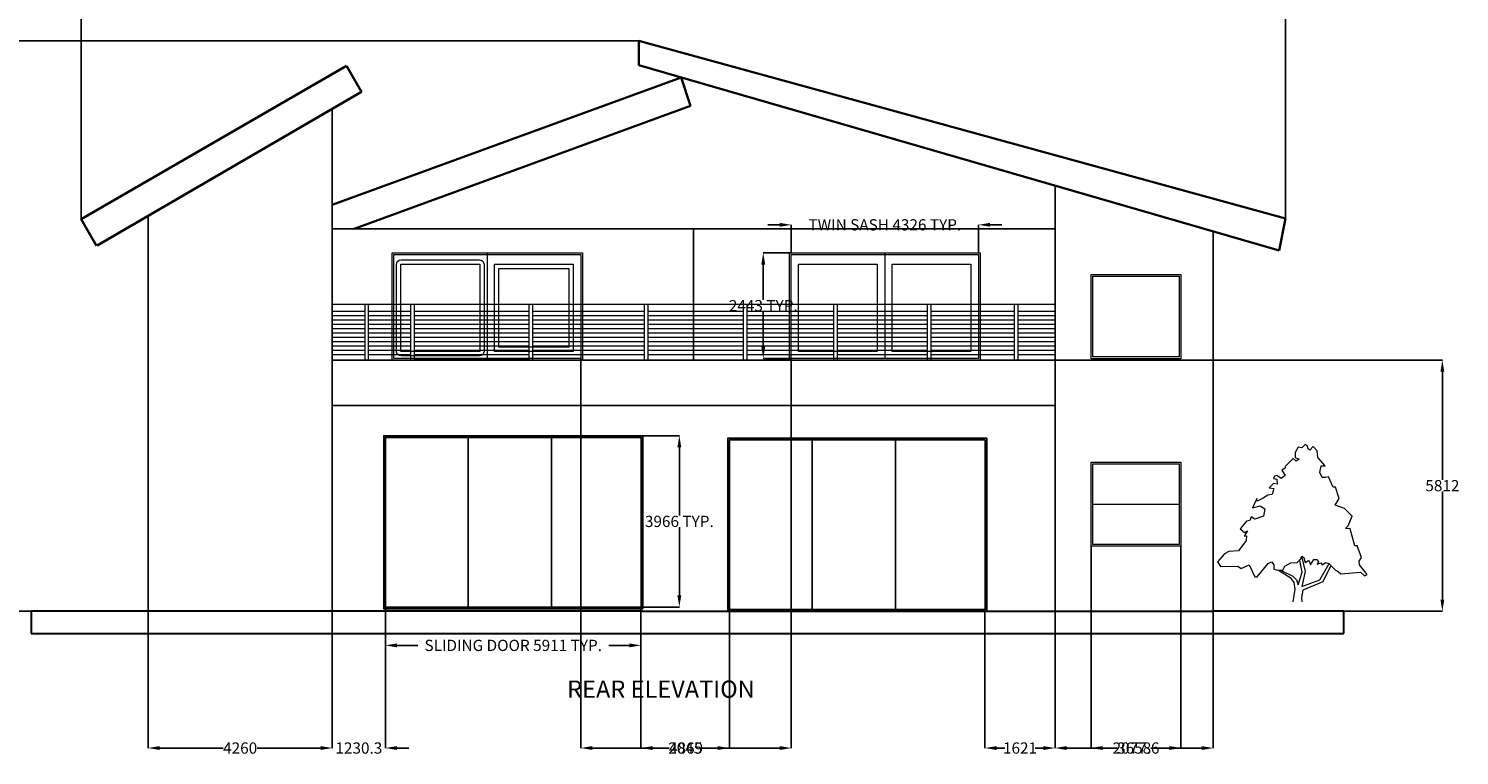
# Model space of a CAD drawing. Units: millimetres. Extents: x 23 to 3809233, y 4 to 290343.
# Tile 5 of 8: x 1915648 to 1948739, y 132658 to 149481. Entities that reach past the tile are written whole.
import ezdxf

# ---------------------------------------------------------------- set-up
doc = ezdxf.new("R2010")
doc.units = ezdxf.units.MM
doc.header["$MEASUREMENT"] = 0
for name, color, linetype, lineweight in [('A-ANNO-DIMS', 2, 'Continuous', 18), ('A-ANNO-TEXT', 7, 'Continuous', 25), ('A-DOOR', 3, 'Continuous', 25), ('A-ELEV', 7, 'Continuous', 25), ('A-ELEV-GRND', 7, 'Continuous', 30), ('A-FLOR-RAIL', 8, 'Continuous', 18), ('A-GLAZ', 4, 'Continuous', 18), ('A-ROOF', 7, 'Continuous', 35), ('L-PLNT', 94, 'Continuous', 13)]:
    doc.layers.add(name, color=color, linetype=linetype, lineweight=lineweight)
doc.styles.get("Standard").update_dxf_attribs({"font": 'arial.ttf'})
doc.dimstyles.get("Standard").update_dxf_attribs({"dimtxt": 260.18, "dimasz": 270.18, "dimexe": 0.18, "dimexo": 0.0625, "dimgap": 0.09, "dimtad": 0, "dimtih": 1, "dimtoh": 1, "dimdec": 0, "dimzin": 0, "dimdsep": 46, "dimtxsty": 'Standard', "dimcen": 0.09, "dimadec": 0, "dimazin": 0, "dimtfac": 1, "dimtdec": 0, "dimtofl": 0, "dimtmove": 0, "dimatfit": 3, "dimfxl": 1, "dimtolj": 1, "dimtzin": 0, "dimarcsym": 0})

# ---------------------------------------------------------------- blocks, each defined once
blk = doc.blocks.new('*U4')
for points in [[(22.0124, 137.721), (18.5475, 141.5624), (15.5282, 138.2446), (13.8028, 139.3505), (13.3714, 142.1153), (11.2148, 143.2214), (8.1954, 140.4564), (4.7447, 141.0094), (2.1567, 136.0326), (2.1567, 131.6088), (5.6074, 129.9499), (3.0193, 128.2909), (0.4313, 130.5029), (-6.9015, 123.3141), (-6.9015, 121.6552), (-9.9208, 119.9963), (-9.0581, 118.3373), (-6.9015, 115.0195), (-10.7835, 112.2546), (-14.6656, 115.0195), (-16.8222, 114.4665), (-17.6849, 112.2546), (-14.6656, 111.7016), (-14.2342, 107.2778), (-17.6065, 107.8307), (-21.5669, 103.9599), (-17.2536, 103.4069), (-18.9789, 97.8771), (-22.8609, 97.3241), (-27.1743, 94.5593), (-32.3504, 91.7944), (-32.7817, 94.0063), (-36.6638, 85.7116), (-29.7624, 87.3705), (-25.449, 84.6056), (-26.743, 77.9699), (-34.507, 75.205), (-37.9578, 77.4169), (-39.2518, 74.099), (-42.2711, 73.5461), (-44.8592, 70.2282), (-47.8786, 66.3574), (-43.9965, 63.0395), (-41.4085, 64.6985), (-44.3346, 59.8898), (-42.2089, 60.1377), (-42.5159, 55.7849), (-49.6039, 46.4502), (-58.2307, 45.8972), (-62.1127, 43.6853), (-68.5828, 36.4966), (-65.9947, 32.0727), (-50.0352, 32.6257), (-47.0159, 30.4138), (-39.6831, 33.7317), (-34.507, 22.6721), (-32.3504, 22.6721), (-22.4296, 34.8376), (-19.4102, 36.4966), (-17.2536, 33.7317), (-17.2536, 29.8608), (-13.8028, 28.7549), (-9.0581, 28.7549), (-7.3328, 32.6257), (-1.7254, 35.3906), (3.8821, 35.9436), (6.4701, 38.1555), (6.9014, 38.7085), (8.1954, 41.4734), (9.9208, 40.3674), (11.2148, 35.9436), (14.2341, 37.6025), (15.0968, 36.4966), (15.9595, 33.7317), (18.9789, 38.7085), (21.9982, 38.7085), (23.2922, 36.4966), (21.9982, 34.2847), (25.4489, 35.3906), (26.743, 33.7317), (29.7623, 35.9436), (32.7817, 34.8376), (38.8204, 28.7549), (41.4084, 27.6489), (43.5651, 25.437), (61.6813, 27.0959), (65.132, 23.7781), (67.7201, 24.884), (60.8186, 33.7317), (60.3873, 37.0495), (62.544, 40.3674), (58.662, 50.874), (56.5053, 50.874), (52.1919, 66.3574), (47.8785, 66.9103), (50.4665, 69.1222), (53.9172, 77.9699), (47.0158, 85.1586), (38.3891, 87.9235), (42.2711, 94.0063)], [(42.2711, 94.0063), (38.8204, 104.5129), (36.6637, 104.5129), (32.3503, 113.9135), (29.7623, 113.3605), (26.743, 113.3605), (24.5862, 117.7844), (25.8802, 123.8671), (29.331, 123.8671), (22.8609, 131.6088), (21.9982, 137.6916)], [(8.1954, 40.3674), (11.2148, 27.6489), (8.1954, 13.8245), (24.5862, 19.9072), (32.7817, 34.2847)], [(-12.9401, 28.7549), (-2.588, 22.1191), (0.8626, 17.6953), (1.7253, 11.6125), (0, 0)], [(-9.9208, 28.2019), (0, 23.2251), (3.4507, 19.9072), (4.7447, 15.4834), (8.6267, 27.0959), (6.4701, 37.6025)], [(34.5071, 33.1787), (27.1743, 18.2483), (9.0581, 10.5066), (7.7641, 3.8708), (8.1954, 0)]]:
    blk.add_lwpolyline(points)
blk = doc.blocks.new('WINDOW-TWIN-SASH-ELEV')
blk.add_line((2163, 2443), (2163, 0))
blk.add_lwpolyline([(0, 2403), (4326, 2403), (4326, 0), (0, 0)], close=True)
for points in [[(165, 2176, -0.414214), (168, 2179), (1985, 2179, -0.414214), (1988, 2176), (1988, 160, -0.414214), (1985, 157), (168, 157, -0.414214), (165, 160)], [(2329, 2176, -0.414214), (2332, 2179), (4148, 2179, -0.414214), (4151, 2176), (4151, 160, -0.414214), (4148, 157), (2332, 157, -0.414214), (2329, 160)]]:
    blk.add_lwpolyline(points, format="xyb", close=True)
blk = doc.blocks.new('SLIDER-THREE-PANEL-ELEV')
for p, q in [((1912, 3966), (1912, 0)), ((3839, 3926), (3839, 0))]:
    blk.add_line(p, q)
blk.add_lwpolyline([(5911, 0), (0, 0), (0, 3926), (5911, 3926)], close=True)
blk = doc.blocks.new('*D44')
at = {"layer": 'A-ANNO-DIMS', "color": 0, "lineweight": -2, "transparency": 16777216}
for p, q in [((1933018, 144939), (1932747, 144939)), ((1933288, 144290), (1933288, 144939)), ((1937614, 144290), (1937614, 144939)), ((1937884, 144939), (1938154, 144939))]:
    blk.add_line(p, q, dxfattribs=at)
at = {"layer": 'A-ANNO-DIMS', "color": 0, "transparency": 16777216}
for points in [[(1933018, 144984), (1933018, 144894), (1933288, 144939)], [(1937884, 144984), (1937884, 144894), (1937614, 144939)]]:
    blk.add_solid(points, dxfattribs=at)
at = {"layer": 'Defpoints', "color": 0, "transparency": 16777216}
for p in [(1937614, 144939), (1933288, 144290), (1937614, 144290)]:
    blk.add_point(p, dxfattribs=at)
at = {"layer": 'A-ANNO-DIMS', "color": 0, "transparency": 16777216, "insert": (1935451, 144939), "char_height": 260.18, "attachment_point": 5}
blk.add_mtext('\\A1;TWIN SASH 4326 TYP.', dxfattribs=at)
blk = doc.blocks.new('*D45')
at = {"layer": 'A-ANNO-DIMS', "color": 0, "lineweight": -2, "transparency": 16777216}
for p, q in [((1933288, 144290), (1932639, 144290)), ((1932639, 144020), (1932639, 143202)), ((1932639, 142117), (1932639, 142935)), ((1933288, 141847), (1932639, 141847))]:
    blk.add_line(p, q, dxfattribs=at)
at = {"layer": 'A-ANNO-DIMS', "color": 0, "transparency": 16777216}
for points in [[(1932594, 144020), (1932684, 144020), (1932639, 144290)], [(1932594, 142117), (1932684, 142117), (1932639, 141847)]]:
    blk.add_solid(points, dxfattribs=at)
at = {"layer": 'Defpoints', "color": 0, "transparency": 16777216}
for p in [(1932639, 144290), (1933288, 144290), (1933288, 141847)]:
    blk.add_point(p, dxfattribs=at)
at = {"layer": 'A-ANNO-DIMS', "color": 0, "transparency": 16777216, "insert": (1932639, 143068), "char_height": 260.18, "attachment_point": 5}
blk.add_mtext('\\A1;2443 TYP.', dxfattribs=at)
blk = doc.blocks.new('*D46')
at = {"layer": 'A-ANNO-DIMS', "color": 0, "lineweight": -2, "transparency": 16777216}
for p, q in [((1923901, 136091), (1923901, 135204)), ((1929811, 136091), (1929811, 135204)), ((1924171, 135204), (1924648, 135204)), ((1929541, 135204), (1929064, 135204))]:
    blk.add_line(p, q, dxfattribs=at)
at = {"layer": 'A-ANNO-DIMS', "color": 0, "transparency": 16777216}
for points in [[(1924171, 135249), (1924171, 135159), (1923901, 135204)], [(1929541, 135249), (1929541, 135159), (1929811, 135204)]]:
    blk.add_solid(points, dxfattribs=at)
at = {"layer": 'Defpoints', "color": 0, "transparency": 16777216}
for p in [(1923901, 136091), (1929811, 136091), (1929811, 135204)]:
    blk.add_point(p, dxfattribs=at)
at = {"layer": 'A-ANNO-DIMS', "color": 0, "transparency": 16777216, "insert": (1926856, 135204), "char_height": 260.18, "attachment_point": 5}
blk.add_mtext('\\A1;SLIDING DOOR 5911 TYP.', dxfattribs=at)
blk = doc.blocks.new('*D47')
at = {"layer": 'A-ANNO-DIMS', "color": 0, "lineweight": -2, "transparency": 16777216}
for p, q in [((1929812, 140056), (1930698, 140056)), ((1930698, 139786), (1930698, 138207)), ((1930698, 136361), (1930698, 137941)), ((1929812, 136091), (1930698, 136091))]:
    blk.add_line(p, q, dxfattribs=at)
at = {"layer": 'A-ANNO-DIMS', "color": 0, "transparency": 16777216}
for points in [[(1930653, 139786), (1930743, 139786), (1930698, 140056)], [(1930653, 136361), (1930743, 136361), (1930698, 136091)]]:
    blk.add_solid(points, dxfattribs=at)
at = {"layer": 'Defpoints', "color": 0, "transparency": 16777216}
for p in [(1929811, 140056), (1930698, 140056), (1929811, 136091)]:
    blk.add_point(p, dxfattribs=at)
at = {"layer": 'A-ANNO-DIMS', "color": 0, "transparency": 16777216, "insert": (1930698, 138074), "char_height": 260.18, "attachment_point": 5}
blk.add_mtext('\\A1;3966 TYP.', dxfattribs=at)
blk = doc.blocks.new('*D116')
at = {"layer": 'A-ANNO-DIMS', "color": 0, "lineweight": -2, "transparency": 16777216}
for p, q in [((1916860, 145073), (1916860, 150759)), ((1917130, 150759), (1930297, 150759)), ((1944447, 150759), (1931281, 150759)), ((1944717, 145084), (1944717, 150759))]:
    blk.add_line(p, q, dxfattribs=at)
at = {"layer": 'A-ANNO-DIMS', "color": 0, "transparency": 16777216}
for points in [[(1917130, 150804), (1917130, 150714), (1916860, 150759)], [(1944447, 150804), (1944447, 150714), (1944717, 150759)]]:
    blk.add_solid(points, dxfattribs=at)
at = {"layer": 'Defpoints', "color": 0, "transparency": 16777216}
for p in [(1944717, 150759), (1916860, 145073), (1944717, 145084)]:
    blk.add_point(p, dxfattribs=at)
at = {"layer": 'A-ANNO-DIMS', "color": 0, "transparency": 16777216, "insert": (1930789, 150759), "char_height": 260.2, "attachment_point": 5}
blk.add_mtext('\\A1;27857', dxfattribs=at)
blk = doc.blocks.new('*D117')
at = {"layer": 'A-ANNO-DIMS', "color": 0, "lineweight": -2, "transparency": 16777216}
for p, q in [((1929762, 149200), (1914150, 149200)), ((1914150, 148930), (1914150, 142731)), ((1914150, 136265), (1914150, 142465)), ((1918411, 135995), (1914150, 135995))]:
    blk.add_line(p, q, dxfattribs=at)
at = {"layer": 'A-ANNO-DIMS', "color": 0, "transparency": 16777216}
for points in [[(1914105, 148930), (1914195, 148930), (1914150, 149200)], [(1914105, 136265), (1914195, 136265), (1914150, 135995)]]:
    blk.add_solid(points, dxfattribs=at)
at = {"layer": 'Defpoints', "color": 0, "transparency": 16777216}
for p in [(1914150, 149200), (1929762, 149200), (1918411, 135995)]:
    blk.add_point(p, dxfattribs=at)
at = {"layer": 'A-ANNO-DIMS', "color": 0, "transparency": 16777216, "insert": (1914150, 142598), "char_height": 260.2, "attachment_point": 5}
blk.add_mtext('\\A1;13205', dxfattribs=at)
blk = doc.blocks.new('*D118')
at = {"layer": 'A-ANNO-DIMS', "color": 0, "lineweight": -2, "transparency": 16777216}
for p, q in [((1918411, 135995), (1918411, 132828)), ((1922671, 135995), (1922671, 132828)), ((1918681, 132828), (1920147, 132828)), ((1922400, 132828), (1920934, 132828))]:
    blk.add_line(p, q, dxfattribs=at)
at = {"layer": 'A-ANNO-DIMS', "color": 0, "transparency": 16777216}
for points in [[(1918681, 132873), (1918681, 132783), (1918411, 132828)], [(1922400, 132873), (1922400, 132783), (1922671, 132828)]]:
    blk.add_solid(points, dxfattribs=at)
at = {"layer": 'Defpoints', "color": 0, "transparency": 16777216}
for p in [(1918411, 135995), (1922671, 135995), (1922671, 132828)]:
    blk.add_point(p, dxfattribs=at)
at = {"layer": 'A-ANNO-DIMS', "color": 0, "transparency": 16777216, "insert": (1920541, 132828), "char_height": 260.2, "attachment_point": 5}
blk.add_mtext('\\A1;4260', dxfattribs=at)
blk = doc.blocks.new('*D119')
at = {"layer": 'A-ANNO-DIMS', "color": 0, "lineweight": -2, "transparency": 16777216}
for p, q in [((1923901, 136091), (1923901, 132828)), ((1922671, 135995), (1922671, 132828)), ((1922400, 132828), (1922130, 132828)), ((1924171, 132828), (1924441, 132828))]:
    blk.add_line(p, q, dxfattribs=at)
at = {"layer": 'A-ANNO-DIMS', "color": 0, "transparency": 16777216}
for points in [[(1922400, 132873), (1922400, 132783), (1922671, 132828)], [(1924171, 132873), (1924171, 132783), (1923901, 132828)]]:
    blk.add_solid(points, dxfattribs=at)
at = {"layer": 'Defpoints', "color": 0, "transparency": 16777216}
for p in [(1923901, 136091), (1922671, 135995), (1923901, 132828)]:
    blk.add_point(p, dxfattribs=at)
at = {"layer": 'A-ANNO-DIMS', "color": 0, "transparency": 16777216, "insert": (1923286, 132828), "char_height": 260.2, "attachment_point": 5}
blk.add_mtext('\\A1;1230.3', dxfattribs=at)
blk = doc.blocks.new('*D120')
at = {"layer": 'A-ANNO-DIMS', "color": 0, "lineweight": -2, "transparency": 16777216}
for p, q in [((1929811, 136091), (1929811, 132828)), ((1931856, 136035), (1931856, 132828)), ((1930082, 132828), (1930442, 132828)), ((1931586, 132828), (1931226, 132828))]:
    blk.add_line(p, q, dxfattribs=at)
at = {"layer": 'A-ANNO-DIMS', "color": 0, "transparency": 16777216}
for points in [[(1930082, 132873), (1930082, 132783), (1929811, 132828)], [(1931586, 132873), (1931586, 132783), (1931856, 132828)]]:
    blk.add_solid(points, dxfattribs=at)
at = {"layer": 'Defpoints', "color": 0, "transparency": 16777216}
for p in [(1929811, 136091), (1931856, 136035), (1931856, 132828)]:
    blk.add_point(p, dxfattribs=at)
at = {"layer": 'A-ANNO-DIMS', "color": 0, "transparency": 16777216, "insert": (1930834, 132828), "char_height": 260.2, "attachment_point": 5}
blk.add_mtext('\\A1;2045', dxfattribs=at)
blk = doc.blocks.new('*D121')
at = {"layer": 'A-ANNO-DIMS', "color": 0, "lineweight": -2, "transparency": 16777216}
for p, q in [((1937767, 136035), (1937767, 132828)), ((1939388, 135995), (1939388, 132828)), ((1938037, 132828), (1938226, 132828)), ((1939118, 132828), (1938929, 132828))]:
    blk.add_line(p, q, dxfattribs=at)
at = {"layer": 'A-ANNO-DIMS', "color": 0, "transparency": 16777216}
for points in [[(1938037, 132873), (1938037, 132783), (1937767, 132828)], [(1939118, 132873), (1939118, 132783), (1939388, 132828)]]:
    blk.add_solid(points, dxfattribs=at)
at = {"layer": 'Defpoints', "color": 0, "transparency": 16777216}
for p in [(1937767, 136035), (1939388, 135995), (1939388, 132828)]:
    blk.add_point(p, dxfattribs=at)
at = {"layer": 'A-ANNO-DIMS', "color": 0, "transparency": 16777216, "insert": (1938577, 132828), "char_height": 260.2, "attachment_point": 5}
blk.add_mtext('\\A1;1621', dxfattribs=at)
blk = doc.blocks.new('*D122')
at = {"layer": 'A-ANNO-DIMS', "color": 0, "lineweight": -2, "transparency": 16777216}
for p, q in [((1939388, 135995), (1939388, 132828)), ((1943046, 135995), (1943046, 132828)), ((1939658, 132828), (1940828, 132828)), ((1942776, 132828), (1941606, 132828))]:
    blk.add_line(p, q, dxfattribs=at)
at = {"layer": 'A-ANNO-DIMS', "color": 0, "transparency": 16777216}
for points in [[(1939658, 132873), (1939658, 132783), (1939388, 132828)], [(1942776, 132873), (1942776, 132783), (1943046, 132828)]]:
    blk.add_solid(points, dxfattribs=at)
at = {"layer": 'Defpoints', "color": 0, "transparency": 16777216}
for p in [(1939388, 135995), (1943046, 135995), (1943046, 132828)]:
    blk.add_point(p, dxfattribs=at)
at = {"layer": 'A-ANNO-DIMS', "color": 0, "transparency": 16777216, "insert": (1941217, 132828), "char_height": 260.2, "attachment_point": 5}
blk.add_mtext('\\A1;3658', dxfattribs=at)
blk = doc.blocks.new('*D123')
at = {"layer": 'A-ANNO-DIMS', "color": 0, "lineweight": -2, "transparency": 16777216}
for p, q in [((1939388, 141807), (1948345, 141807)), ((1948345, 141537), (1948345, 139034)), ((1948345, 136265), (1948345, 138768)), ((1939388, 135995), (1948345, 135995))]:
    blk.add_line(p, q, dxfattribs=at)
at = {"layer": 'A-ANNO-DIMS', "color": 0, "transparency": 16777216}
for points in [[(1948300, 141537), (1948390, 141537), (1948345, 141807)], [(1948300, 136265), (1948390, 136265), (1948345, 135995)]]:
    blk.add_solid(points, dxfattribs=at)
at = {"layer": 'Defpoints', "color": 0, "transparency": 16777216}
for p in [(1939388, 141807), (1948345, 141807), (1939388, 135995)]:
    blk.add_point(p, dxfattribs=at)
at = {"layer": 'A-ANNO-DIMS', "color": 0, "transparency": 16777216, "insert": (1948345, 138901), "char_height": 260.2, "attachment_point": 5}
blk.add_mtext('\\A1;5812', dxfattribs=at)
blk = doc.blocks.new('*D124')
at = {"layer": 'A-ANNO-DIMS', "color": 0, "lineweight": -2, "transparency": 16777216}
for p, q in [((1928419, 141847), (1928419, 132828)), ((1933288, 141847), (1933288, 132828)), ((1928689, 132828), (1930459, 132828)), ((1933018, 132828), (1931247, 132828))]:
    blk.add_line(p, q, dxfattribs=at)
at = {"layer": 'A-ANNO-DIMS', "color": 0, "transparency": 16777216}
for points in [[(1928689, 132873), (1928689, 132783), (1928419, 132828)], [(1933018, 132873), (1933018, 132783), (1933288, 132828)]]:
    blk.add_solid(points, dxfattribs=at)
at = {"layer": 'Defpoints', "color": 0, "transparency": 16777216}
for p in [(1928419, 141847), (1933288, 141847), (1933288, 132828)]:
    blk.add_point(p, dxfattribs=at)
at = {"layer": 'A-ANNO-DIMS', "color": 0, "transparency": 16777216, "insert": (1930853, 132828), "char_height": 260.2, "attachment_point": 5}
blk.add_mtext('\\A1;4869', dxfattribs=at)
blk = doc.blocks.new('*D125')
at = {"layer": 'A-ANNO-DIMS', "color": 0, "lineweight": -2, "transparency": 16777216}
for p, q in [((1940221, 137500), (1940221, 132828)), ((1942298, 137501), (1942298, 132828)), ((1940491, 132828), (1940717, 132828)), ((1942028, 132828), (1941802, 132828))]:
    blk.add_line(p, q, dxfattribs=at)
at = {"layer": 'A-ANNO-DIMS', "color": 0, "transparency": 16777216}
for points in [[(1940491, 132873), (1940491, 132783), (1940221, 132828)], [(1942028, 132873), (1942028, 132783), (1942298, 132828)]]:
    blk.add_solid(points, dxfattribs=at)
at = {"layer": 'Defpoints', "color": 0, "transparency": 16777216}
for p in [(1940221, 137500), (1942298, 137501), (1942298, 132828)]:
    blk.add_point(p, dxfattribs=at)
at = {"layer": 'A-ANNO-DIMS', "color": 0, "transparency": 16777216, "insert": (1941260, 132828), "char_height": 260.2, "attachment_point": 5}
blk.add_mtext('\\A1;2077.6', dxfattribs=at)

msp = doc.modelspace()

# ---------------------------------------------------------------- linework, layer by layer
at = {"layer": 'A-DOOR'}
for points in [[(1929851.48, 136053.678, -0.414213562), (1929848.48, 136050.678), (1923863.823, 136050.678, -0.414213562), (1923860.823, 136053.678), (1923860.823, 140053.392, -0.414213562), (1923863.823, 140056.392), (1929848.48, 140056.392, -0.414213562), (1929851.48, 140053.392)], [(1937806.946, 135998.166, -0.414213562), (1937803.946, 135995.166), (1931819.29, 135995.166, -0.414213562), (1931816.29, 135998.166), (1931816.29, 139997.881, -0.414213562), (1931819.29, 140000.881), (1937803.946, 140000.881, -0.414213562), (1937806.946, 139997.881)]]:
    msp.add_lwpolyline(points, format="xyb", close=True, dxfattribs=at)
at = {"layer": 'A-ELEV'}
for p, q in [((1922670.515, 135995.166), (1922670.515, 147619.145)), ((1939387.964, 145848.069), (1939387.964, 135995.166)), ((1918410.662, 135995.166), (1918410.662, 145140.935)), ((1939387.964, 144846.348), (1922670.515, 144846.348)), ((1931029.239, 144846.348), (1931029.239, 141807.156)), ((1943046.284, 135995.166), (1943046.284, 144785.585)), ((1922670.515, 141807.156), (1939387.964, 141807.156)), ((1922670.515, 140754.714), (1939387.964, 140754.714))]:
    msp.add_line(p, q, dxfattribs=at)
at = {"layer": 'A-ELEV-GRND'}
for p, q in [((1918410.662, 135995.166), (1915708.258, 135995.166)), ((1915708.258, 135995.166), (1915708.258, 135482.58)), ((1919885.432, 135995.166), (1918410.662, 135995.166)), ((1926477.421, 135995.166), (1919885.432, 135995.166)), ((1929846.284, 135995.166), (1926477.421, 135995.166)), ((1929846.284, 135995.166), (1943046.284, 135995.166)), ((1946066.446, 135995.166), (1943046.284, 135995.166)), ((1946066.446, 135482.58), (1946066.446, 135995.166)), ((1915708.258, 135482.58), (1946066.446, 135482.58))]:
    msp.add_line(p, q, dxfattribs=at)
at = {"layer": 'A-FLOR-RAIL'}
for p, q in [((1922670.515, 143103.299), (1939387.964, 143103.299)), ((1923420.547, 143103.299), (1923420.547, 141807.156)), ((1923502.129, 143103.299), (1923502.129, 141807.156)), ((1924481.889, 143103.299), (1924481.889, 141807.156)), ((1924563.471, 143103.299), (1924563.471, 141807.156)), ((1927220.711, 143103.299), (1927220.711, 141807.156)), ((1927302.293, 143103.299), (1927302.293, 141807.156)), ((1929886.792, 143103.299), (1929886.792, 141807.156)), ((1929968.374, 143103.299), (1929968.374, 141807.156)), ((1932174.846, 143103.299), (1932174.846, 141807.156)), ((1932256.428, 143103.299), (1932256.428, 141807.156)), ((1934263.939, 143103.299), (1934263.939, 141807.156)), ((1934345.521, 143103.299), (1934345.521, 141807.156)), ((1936432.618, 143103.299), (1936432.618, 141807.156)), ((1936514.2, 143103.299), (1936514.2, 141807.156)), ((1938442.129, 143103.299), (1938442.129, 141807.156)), ((1938523.711, 143103.299), (1938523.711, 141807.156)), ((1922670.515, 142937.436), (1923420.547, 142937.436)), ((1922670.515, 142837.436), (1923420.547, 142837.436)), ((1922670.515, 142737.436), (1923420.547, 142737.436)), ((1922670.515, 142637.436), (1923420.547, 142637.436)), ((1923502.129, 142937.436), (1924481.889, 142937.436)), ((1923502.129, 142837.436), (1924481.889, 142837.436)), ((1923502.129, 142737.436), (1924481.889, 142737.436)), ((1923502.129, 142637.436), (1924481.889, 142637.436)), ((1924563.471, 142937.436), (1927220.711, 142937.436)), ((1924563.471, 142837.436), (1927220.711, 142837.436)), ((1924563.471, 142737.436), (1927220.711, 142737.436)), ((1924563.471, 142637.436), (1927220.711, 142637.436)), ((1927302.293, 142937.436), (1929886.792, 142937.436)), ((1927302.293, 142837.436), (1929886.792, 142837.436)), ((1927302.293, 142737.436), (1929886.792, 142737.436)), ((1927302.293, 142637.436), (1929886.792, 142637.436)), ((1929968.374, 142937.436), (1932174.846, 142937.436)), ((1929968.374, 142837.436), (1932174.846, 142837.436)), ((1929968.374, 142737.436), (1932174.846, 142737.436)), ((1929968.374, 142637.436), (1932174.846, 142637.436)), ((1932256.428, 142937.436), (1934263.939, 142937.436)), ((1932256.428, 142837.436), (1934263.939, 142837.436)), ((1932256.428, 142737.436), (1934263.939, 142737.436)), ((1932256.428, 142637.436), (1934263.939, 142637.436)), ((1934345.521, 142937.436), (1936432.618, 142937.436)), ((1934345.521, 142837.436), (1936432.618, 142837.436)), ((1934345.521, 142737.436), (1936432.618, 142737.436)), ((1934345.521, 142637.436), (1936432.618, 142637.436)), ((1936514.2, 142937.436), (1938442.129, 142937.436)), ((1936514.2, 142837.436), (1938442.129, 142837.436)), ((1936514.2, 142737.436), (1938442.129, 142737.436)), ((1936514.2, 142637.436), (1938442.129, 142637.436)), ((1938523.711, 142937.436), (1939387.964, 142937.436)), ((1938523.711, 142837.436), (1939387.964, 142837.436)), ((1938523.711, 142737.436), (1939387.964, 142737.436)), ((1938523.711, 142637.436), (1939387.964, 142637.436)), ((1922670.515, 142537.436), (1923420.547, 142537.436)), ((1922670.515, 142437.436), (1923420.547, 142437.436)), ((1922670.515, 142337.436), (1923420.547, 142337.436)), ((1923502.129, 142537.436), (1924481.889, 142537.436)), ((1923502.129, 142437.436), (1924481.889, 142437.436)), ((1923502.129, 142337.436), (1924481.889, 142337.436)), ((1924563.471, 142537.436), (1927220.711, 142537.436)), ((1924563.471, 142437.436), (1927220.711, 142437.436)), ((1924563.471, 142337.436), (1927220.711, 142337.436)), ((1927302.293, 142537.436), (1929886.792, 142537.436)), ((1927302.293, 142437.436), (1929886.792, 142437.436)), ((1927302.293, 142337.436), (1929886.792, 142337.436)), ((1929968.374, 142537.436), (1932174.846, 142537.436)), ((1929968.374, 142437.436), (1932174.846, 142437.436)), ((1929968.374, 142337.436), (1932174.846, 142337.436)), ((1932256.428, 142537.436), (1934263.939, 142537.436)), ((1932256.428, 142437.436), (1934263.939, 142437.436)), ((1932256.428, 142337.436), (1934263.939, 142337.436)), ((1934345.521, 142537.436), (1936432.618, 142537.436)), ((1934345.521, 142437.436), (1936432.618, 142437.436)), ((1934345.521, 142337.436), (1936432.618, 142337.436)), ((1936514.2, 142537.436), (1938442.129, 142537.436)), ((1936514.2, 142437.436), (1938442.129, 142437.436)), ((1936514.2, 142337.436), (1938442.129, 142337.436)), ((1938523.711, 142537.436), (1939387.964, 142537.436)), ((1938523.711, 142437.436), (1939387.964, 142437.436)), ((1938523.711, 142337.436), (1939387.964, 142337.436)), ((1922670.515, 142237.436), (1923420.547, 142237.436)), ((1922670.515, 142137.436), (1923420.547, 142137.436)), ((1922670.515, 142037.436), (1923420.547, 142037.436)), ((1923502.129, 142237.436), (1924481.889, 142237.436)), ((1923502.129, 142137.436), (1924481.889, 142137.436)), ((1923502.129, 142037.436), (1924481.889, 142037.436)), ((1923502.129, 142037.436), (1924481.889, 142037.436)), ((1924563.471, 142237.436), (1927220.711, 142237.436)), ((1924563.471, 142137.436), (1927220.711, 142137.436)), ((1924563.471, 142037.436), (1927220.711, 142037.436)), ((1927302.293, 142237.436), (1929886.792, 142237.436)), ((1927302.293, 142137.436), (1929886.792, 142137.436)), ((1927302.293, 142037.436), (1929886.792, 142037.436)), ((1929968.374, 142237.436), (1932174.846, 142237.436)), ((1929968.374, 142137.436), (1932174.846, 142137.436)), ((1929968.374, 142037.436), (1932174.846, 142037.436)), ((1932256.428, 142237.436), (1934263.939, 142237.436)), ((1932256.428, 142137.436), (1934263.939, 142137.436)), ((1932256.428, 142037.436), (1934263.939, 142037.436)), ((1934345.521, 142237.436), (1936432.618, 142237.436)), ((1934345.521, 142137.436), (1936432.618, 142137.436)), ((1934345.521, 142037.436), (1936432.618, 142037.436)), ((1936514.2, 142237.436), (1938442.129, 142237.436)), ((1936514.2, 142137.436), (1938442.129, 142137.436)), ((1936514.2, 142037.436), (1938442.129, 142037.436)), ((1938523.711, 142237.436), (1939387.964, 142237.436)), ((1938523.711, 142137.436), (1939387.964, 142137.436)), ((1938523.711, 142037.436), (1939387.964, 142037.436)), ((1922670.515, 141937.436), (1923420.547, 141937.436)), ((1923502.129, 141937.436), (1924481.889, 141937.436)), ((1924563.471, 141937.436), (1927220.711, 141937.436)), ((1924563.471, 141837.436), (1927220.711, 141837.436)), ((1927302.293, 141937.436), (1929886.792, 141937.436)), ((1929968.374, 141937.436), (1932174.846, 141937.436)), ((1932256.428, 141937.436), (1934263.939, 141937.436)), ((1934345.521, 141937.436), (1936432.618, 141937.436)), ((1936514.2, 141937.436), (1938442.129, 141937.436)), ((1938523.711, 141937.436), (1939387.964, 141937.436))]:
    msp.add_line(p, q, dxfattribs=at)
msp.add_lwpolyline([(1924158.016, 144023.421, -0.414213562), (1924261.016, 144126.421), (1926077.545, 144126.421, -0.414213562), (1926180.545, 144023.421), (1926180.545, 142006.9, -0.414213562), (1926077.545, 141903.9), (1924261.016, 141903.9, -0.414213562), (1924158.016, 142006.9)], format="xyb", close=True, dxfattribs=at)
for points in [[(1926421.396, 144026.421), (1928243.925, 144026.421), (1928243.925, 142003.9), (1926421.396, 142003.9)], [(1926521.396, 143926.421), (1928143.925, 143926.421), (1928143.925, 142103.9), (1926521.396, 142103.9)]]:
    msp.add_lwpolyline(points, close=True, dxfattribs=at)
at = {"layer": 'A-GLAZ'}
msp.add_line((1940259.956, 138473.775), (1942258.617, 138473.775), dxfattribs=at)
for points in [[(1924052.673, 144286.834, -0.414213562), (1924055.673, 144289.834), (1928456.001, 144289.834, -0.414213562), (1928459.001, 144286.834), (1928459.001, 141810.156, -0.414213562), (1928456.001, 141807.156), (1924055.673, 141807.156, -0.414213562), (1924052.673, 141810.156)], [(1933247.747, 144286.834, -0.414213562), (1933250.747, 144289.834), (1937651.075, 144289.834, -0.414213562), (1937654.075, 144286.834), (1937654.075, 141810.156, -0.414213562), (1937651.075, 141807.156), (1933250.747, 141807.156, -0.414213562), (1933247.747, 141810.156)], [(1940219.956, 143787.119, -0.414213562), (1940222.956, 143790.119), (1942295.617, 143790.119, -0.414213562), (1942298.617, 143787.119), (1942298.617, 141843.627, -0.414213562), (1942295.617, 141840.627), (1940222.956, 141840.627, -0.414213562), (1940219.956, 141843.627)], [(1940219.956, 139445.521, -0.414213562), (1940222.956, 139448.521), (1942295.617, 139448.521, -0.414213562), (1942298.617, 139445.521), (1942298.617, 137502.029, -0.414213562), (1942295.617, 137499.029), (1940222.956, 137499.029, -0.414213562), (1940219.956, 137502.029)]]:
    msp.add_lwpolyline(points, format="xyb", close=True, dxfattribs=at)
for points in [[(1940259.956, 143750.119), (1942258.617, 143750.119), (1942258.617, 141880.627), (1940259.956, 141880.627)], [(1940259.956, 139408.521), (1942258.617, 139408.521), (1942258.617, 137539.029), (1940259.956, 137539.029)]]:
    msp.add_lwpolyline(points, close=True, dxfattribs=at)
at = {"layer": 'A-ROOF'}
for p, q in [((1929762.389, 148632.871), (1929762.389, 149200.29)), ((1929762.389, 149200.29), (1944717.474, 145083.818)), ((1923001.157, 148618.439), (1916859.981, 145072.83)), ((1923350.186, 148013.903), (1923001.157, 148618.439)), ((1944573.273, 144343.337), (1929762.389, 148632.871)), ((1930736.899, 148350.633), (1922670.515, 145401.797)), ((1930953.441, 147691.903), (1930736.899, 148350.633)), ((1917236.917, 144463.273), (1923350.186, 148013.903)), ((1923175.061, 144846.348), (1930953.441, 147691.903)), ((1916859.981, 145072.83), (1917219.793, 144453.327)), ((1944717.474, 145083.818), (1944573.273, 144343.337)), ((1943046.284, 144785.585), (1943046.284, 144785.585))]:
    msp.add_line(p, q, dxfattribs=at)

# ---------------------------------------------------------------- block references
at = {"layer": 'A-DOOR'}
for p in [(1923900.824, 136090.677), (1931856.29, 136035.166)]:
    msp.add_blockref('SLIDER-THREE-PANEL-ELEV', p, dxfattribs=at)
at = {"layer": 'A-GLAZ'}
for p in [(1924092.673, 141847.156), (1933287.747, 141847.156)]:
    msp.add_blockref('WINDOW-TWIN-SASH-ELEV', p, dxfattribs=at)
at = {"layer": 'L-PLNT', "xscale": 25.4, "yscale": 25.4, "zscale": 25.4}
msp.add_blockref('*U4', (1944887.077, 136212.712), dxfattribs=at)

# ---------------------------------------------------------------- texts
at = {"layer": 'A-ANNO-TEXT', "insert": (1928102.441, 134391.388), "char_height": 400, "attachment_point": 1}
msp.add_mtext_dynamic_manual_height_columns('REAR ELEVATION', width=8410.77875, gutter_width=1, heights=[307.465], dxfattribs=at)

# ---------------------------------------------------------------- dimensions: what is measured, and where the dimension line sits
at = {"layer": 'A-ANNO-DIMS'}
for base, p1, p2, override, picture, middle in [((1944717.474, 150758.79), (1916859.981, 145072.83), (1944717.474, 145083.818), {"dimdec": 0, "dimlfac": 1, "dimrnd": 0, "dimzin": 0, "dimdsep": 46, "dimlunit": 2}, '*D116', (1930788.728, 150758.79)), ((1933287.747, 132828.282), (1928419.001, 141847.156), (1933287.747, 141847.156), {"dimdec": 0, "dimlfac": 1, "dimrnd": 0, "dimzin": 0, "dimdsep": 46, "dimlunit": 2}, '*D124', (1930853.374, 132828.282)), ((1942298.388, 132828.282), (1940220.835, 137499.907), (1942298.388, 137500.88), {"dimdec": 1, "dimlfac": 1, "dimrnd": 0, "dimzin": 0, "dimdsep": 46, "dimlunit": 2}, '*D125', (1941259.612, 132828.282)), ((1923900.823, 132828.282), (1922670.515, 135995.166), (1923900.823, 136090.678), {"dimdec": 1, "dimlfac": 1, "dimrnd": 0, "dimzin": 0, "dimdsep": 46, "dimlunit": 2}, '*D119', (1923285.669, 132828.282)), ((1931856.29, 132828.282), (1929811.48, 136090.678), (1931856.29, 136035.166), {"dimdec": 0, "dimlfac": 1, "dimrnd": 0, "dimzin": 0, "dimdsep": 46, "dimlunit": 2}, '*D120', (1930833.885, 132828.282)), ((1939387.964, 132828.282), (1937766.946, 136035.166), (1939387.964, 135995.166), {"dimdec": 0, "dimlfac": 1, "dimrnd": 0, "dimzin": 0, "dimdsep": 46, "dimlunit": 2}, '*D121', (1938577.455, 132828.282)), ((1922670.515, 132828.282), (1918410.662, 135995.166), (1922670.515, 135995.166), {"dimdec": 0, "dimlfac": 1, "dimrnd": 0, "dimzin": 0, "dimdsep": 46, "dimlunit": 2}, '*D118', (1920540.589, 132828.282)), ((1943046.284, 132828.282), (1939387.964, 135995.166), (1943046.284, 135995.166), {"dimdec": 0, "dimlfac": 1, "dimrnd": 0, "dimzin": 0, "dimdsep": 46, "dimlunit": 2}, '*D122', (1941217.124, 132828.282))]:
    dim = msp.add_linear_dim(base=base, p1=p1, p2=p2, dimstyle='Standard', override=override, dxfattribs=at)
    dim.commit()
    dim.dimension.update_dxf_attribs({"geometry": picture, "text_midpoint": middle})
for base, p1, p2, picture, middle in [((1914149.758, 149200.29), (1918410.662, 135995.166), (1929762.389, 149200.29), '*D117', (1914149.758, 142597.728)), ((1948344.634, 141807.156), (1939387.964, 135995.166), (1939387.964, 141807.156), '*D123', (1948344.634, 138901.161))]:
    dim = msp.add_linear_dim(base=base, p1=p1, p2=p2, angle=90, dimstyle='Standard', override={"dimdec": 0, "dimlfac": 1, "dimrnd": 0, "dimzin": 0, "dimdsep": 46, "dimlunit": 2}, dxfattribs=at)
    dim.commit()
    dim.dimension.update_dxf_attribs({"geometry": picture, "text_midpoint": middle})
for base, p1, p2, text, picture, middle in [((1937614.075, 144938.783), (1933287.747, 144289.834), (1937614.075, 144289.834), 'TWIN SASH <> TYP.', '*D44', (1935450.911, 144938.783)), ((1929811.48, 135204.079), (1923900.823, 136090.678), (1929811.48, 136090.678), 'SLIDING DOOR <> TYP.', '*D46', (1926856.152, 135204.079))]:
    dim = msp.add_linear_dim(base=base, p1=p1, p2=p2, text=text, dimstyle='Standard', override={"dimdec": 0, "dimlfac": 1, "dimrnd": 0, "dimzin": 0, "dimdsep": 46, "dimlunit": 2}, dxfattribs=at)
    dim.commit()
    dim.dimension.update_dxf_attribs({"geometry": picture, "text_midpoint": middle})
for base, p1, p2, picture, middle in [((1932638.798, 144289.834), (1933287.747, 141847.156), (1933287.747, 144289.834), '*D45', (1932638.798, 143068.495)), ((1930698.078, 140056.392), (1929811.48, 136090.678), (1929811.48, 140056.392), '*D47', (1930698.078, 138073.535))]:
    dim = msp.add_linear_dim(base=base, p1=p1, p2=p2, angle=90, text='<> TYP.', dimstyle='Standard', override={"dimdec": 0, "dimlfac": 1, "dimrnd": 0, "dimzin": 0, "dimdsep": 46, "dimlunit": 2}, dxfattribs=at)
    dim.commit()
    dim.dimension.update_dxf_attribs({"geometry": picture, "text_midpoint": middle})

doc.saveas('drawing.dxf')
